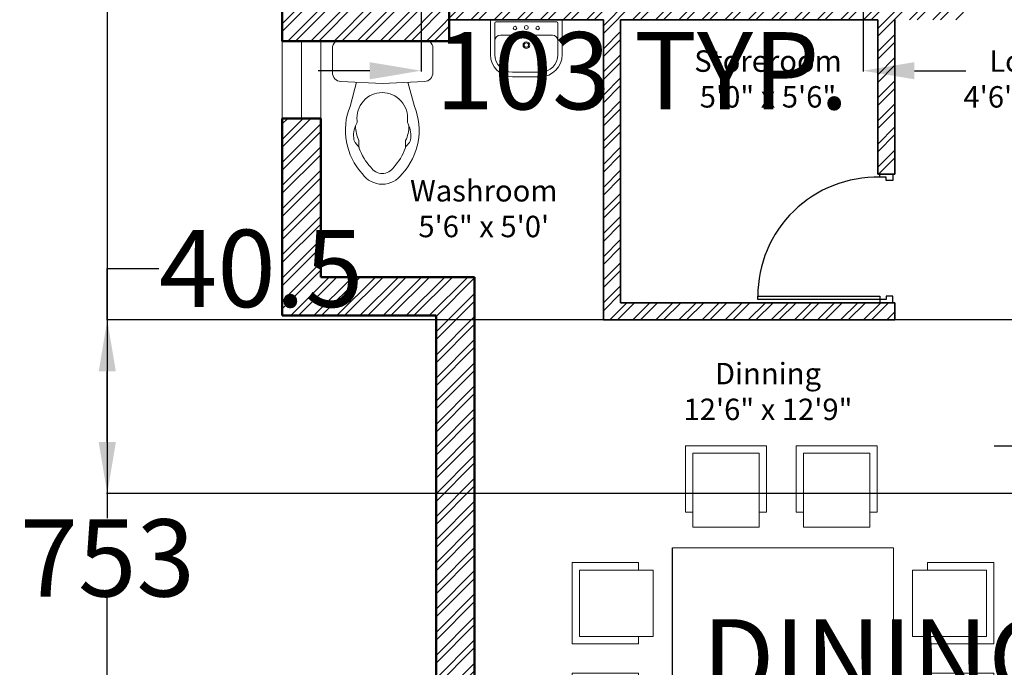
# Model space of a CAD drawing. Units: inches. Extents: x -90 to 536, y -553 to 299.
# Tile 15 of 27: x -23 to 207, y -153 to -2. Entities that reach past the tile are written whole.
import ezdxf

# ---------------------------------------------------------------- set-up
doc = ezdxf.new("R2010")
doc.units = ezdxf.units.IN
for name, color, linetype, lineweight in [('A-ANNO-DIMS', 2, 'Continuous', 18), ('A-AREA-IDEN', 7, 'Continuous', 18), ('A-DOOR', 4, 'Continuous', 25), ('A-FLOR-FIXT', 8, 'Continuous', 18), ('A-GLAZ', 4, 'Continuous', 18), ('A-WALL-PATT', 252, 'Continuous', 13), ('Furniture', 2, 'Continuous', 18), ('Inner Wall', 5, 'Continuous', 35), ('Outer Wall', 1, 'Continuous', 50)]:
    doc.layers.add(name, color=color, linetype=linetype, lineweight=lineweight)
doc.styles.get("Standard").update_dxf_attribs({"font": 'arial.ttf'})
doc.dimstyles.get("Standard").update_dxf_attribs({"dimtxt": 18, "dimasz": 12, "dimexe": 0.18, "dimexo": 0.0625, "dimgap": 0.09, "dimtad": 0, "dimtih": 1, "dimtoh": 1, "dimdec": 0, "dimzin": 0, "dimdsep": 46, "dimlunit": 3, "dimtxsty": 'Standard', "dimcen": 0.09, "dimadec": 0, "dimazin": 0, "dimtfac": 1, "dimtdec": 0, "dimtofl": 0, "dimtmove": 0, "dimatfit": 3, "dimfxl": 1, "dimtolj": 1, "dimtzin": 0, "dimarcsym": 0})

# ---------------------------------------------------------------- blocks, each defined once
blk = doc.blocks.new('A$C1308471B')
at = {"ltscale": 20}
for p, q in [((0.0354, 0.4793), (0.1495, 0.4793)), ((0, 0.4607), (0, 0.0186)), ((0.2013, 0.2397), (0.1923, 0.4384)), ((0.1957, 0.3639), (0.3109, 0.3953)), ((0.5021, 0.3528), (0.4724, 0.3528)), ((0.4982, 0.3575), (0.4822, 0.3709)), ((0.2013, 0.2397), (0.1923, 0.0409)), ((0.1959, 0.1193), (0.3109, 0.0879)), ((0.5021, 0.1304), (0.4724, 0.1304)), ((0.4982, 0.1257), (0.4822, 0.1123)), ((0.0354, 0), (0.1495, 0))]:
    blk.add_line(p, q, dxfattribs=at)
for centre, radius, start, end in [((0.0354, 0.4328), 0.0465, 90, 136.5269), ((0.1495, 0.4365), 0.0429, 2.5755, 90), ((0.006, 0.4607), 0.006, 136.5269, 180), ((0.4248, 0.1104), 0.3068, 47.4135, 111.7924), ((0.4494, 0.2636), 0.1148, 79.3968, 118.5742), ((0.4658, 0.3513), 0.0255, 50, 79.3968), ((0.3654, 0.2416), 0.1206, 83.3523, 180), ((0.3823, 0.3868), 0.0255, 263.3523, 298.5742), ((0.405, 0.2159), 0.153, 63.502, 90.4522), ((0.5146, 0.377), 0.0255, 230, 251.3881), ((0.5021, 0.3273), 0.0255, 70.3751, 90), ((0.4248, 0.1104), 0.2558, 46.612, 70.3751), ((0.5654, 0.2416), 0.116, 0, 54.7115), ((0.5654, 0.2416), 0.065, 0, 57.2974), ((0.3654, 0.2416), 0.1206, 180, 276.6477), ((0.5654, 0.2416), 0.065, 302.7026, 0), ((0.5654, 0.2416), 0.116, 305.2885, 0), ((0.4248, 0.3728), 0.3068, 248.2076, 312.5865), ((0.4248, 0.3728), 0.2558, 289.6249, 313.388), ((0.3823, 0.0964), 0.0255, 61.4258, 96.6477), ((0.4494, 0.2196), 0.1148, 241.4258, 280.6032), ((0.405, 0.2673), 0.153, 269.5478, 296.498), ((0.4658, 0.1319), 0.0255, 280.6032, 310), ((0.5146, 0.1062), 0.0255, 108.6119, 130), ((0.5021, 0.1559), 0.0255, 270, 289.6249), ((0.006, 0.0186), 0.006, 180, 223.4731), ((0.0354, 0.0465), 0.0465, 223.4731, 270), ((0.1495, 0.0429), 0.0429, 270, 357.4245)]:
    blk.add_arc(centre, radius, start, end, dxfattribs=at)
blk = doc.blocks.new('A$C57EA129C')
for p, q in [((0, 0.4428), (0, 0.1782)), ((0.016, 0.4589), (0.5631, 0.4589)), ((0.0356, 0.4321), (0.0356, 0.2896)), ((0.0445, 0.441), (0.5346, 0.441)), ((0.5435, 0.4321), (0.5435, 0.2896)), ((0.5791, 0.4428), (0.5791, 0.1782)), ((0.0802, 0.3341), (0.499, 0.3341)), ((0.0356, 0.2896), (0.0356, 0.1782)), ((0.5435, 0.2896), (0.5435, 0.1782)), ((0.1782, 0.0356), (0.4009, 0.0356)), ((0.1782, 0), (0.4009, 0))]:
    blk.add_line(p, q)
for centre, radius in [((0.1982, 0.392), 0.0143), ((0.2896, 0.3965), 0.0156), ((0.3809, 0.392), 0.0143), ((0.2896, 0.2545), 0.0267), ((0.2896, 0.2545), 0.0178)]:
    blk.add_circle(centre, radius)
for centre, radius, start, end in [((0.016, 0.4428), 0.016, 90, 180), ((0.0445, 0.4321), 0.00891, 90, 180), ((0.5346, 0.4321), 0.00891, 0, 90), ((0.5631, 0.4428), 0.016, 0, 90), ((0.0802, 0.2896), 0.0445, 90, 180), ((0.499, 0.2896), 0.0445, 0, 90), ((0.1782, 0.1782), 0.1782, 180, 270), ((0.1782, 0.1782), 0.1426, 180, 270), ((0.4009, 0.1782), 0.1782, 270, 0), ((0.4009, 0.1782), 0.1426, 270, 0)]:
    blk.add_arc(centre, radius, start, end)
blk = doc.blocks.new('A$C010165D4')
for p, q in [((0.7697, 2.4221), (0.7697, 2.8721)), ((0.7697, 2.8721), (1.3197, 2.8721)), ((1.3197, 2.8721), (1.3197, 2.4221)), ((1.5197, 2.4221), (1.5197, 2.8721)), ((1.5197, 2.8721), (2.0697, 2.8721)), ((2.0697, 2.8721), (2.0697, 2.4221)), ((0.8197, 2.8221), (0.8197, 2.3221)), ((1.2697, 2.8221), (0.8197, 2.8221)), ((1.2697, 2.3221), (1.2697, 2.8221)), ((1.5697, 2.8221), (1.5697, 2.3221)), ((2.0197, 2.8221), (1.5697, 2.8221)), ((2.0197, 2.3221), (2.0197, 2.8221)), ((0.8197, 2.4221), (0.7697, 2.4221)), ((1.3197, 2.4221), (1.2697, 2.4221)), ((1.5697, 2.4221), (1.5197, 2.4221)), ((2.0697, 2.4221), (2.0197, 2.4221)), ((1.2697, 2.3221), (0.8197, 2.3221)), ((2.0197, 2.3221), (1.5697, 2.3221)), ((0.6788, 2.1805), (0.6788, 0.6805)), ((0.6811, 0.6805), (0.6811, 2.1805)), ((0.6811, 2.1805), (2.1811, 2.1805)), ((2.1811, 2.1805), (2.1811, 0.6805)), ((0, 1.531), (0, 2.081)), ((0, 2.081), (0.45, 2.081)), ((0.45, 2.081), (0.45, 2.031)), ((2.8599, 2.081), (2.4099, 2.081)), ((2.4099, 2.081), (2.4099, 2.031)), ((2.8599, 1.531), (2.8599, 2.081)), ((0.05, 2.031), (0.05, 1.581)), ((0.55, 2.031), (0.05, 2.031)), ((0.55, 2.031), (0.55, 1.581)), ((2.3099, 2.031), (2.8099, 2.031)), ((2.3099, 2.031), (2.3099, 1.581)), ((2.8099, 2.031), (2.8099, 1.581)), ((0.05, 1.581), (0.55, 1.581)), ((0.45, 1.581), (0.45, 1.531)), ((2.8099, 1.581), (2.3099, 1.581)), ((2.4099, 1.581), (2.4099, 1.531)), ((0.45, 1.531), (0, 1.531)), ((2.4099, 1.531), (2.8599, 1.531)), ((0, 0.781), (0, 1.331)), ((0, 1.331), (0.45, 1.331)), ((0.05, 1.281), (0.05, 0.831)), ((0.55, 1.281), (0.05, 1.281)), ((0.45, 1.331), (0.45, 1.281)), ((0.55, 1.281), (0.55, 0.831)), ((2.3099, 1.281), (2.8099, 1.281)), ((2.3099, 1.281), (2.3099, 0.831)), ((2.4099, 1.331), (2.4099, 1.281)), ((2.8599, 1.331), (2.4099, 1.331)), ((2.8099, 1.281), (2.8099, 0.831)), ((2.8599, 0.781), (2.8599, 1.331)), ((0.05, 0.831), (0.55, 0.831)), ((0.45, 0.831), (0.45, 0.781)), ((2.8099, 0.831), (2.3099, 0.831)), ((2.4099, 0.831), (2.4099, 0.781)), ((0.45, 0.781), (0, 0.781)), ((2.4099, 0.781), (2.8599, 0.781)), ((2.1811, 0.6805), (0.6811, 0.6805)), ((0.8197, 0.05), (0.8197, 0.55)), ((1.2697, 0.55), (0.8197, 0.55)), ((1.2697, 0.55), (1.2697, 0.05)), ((1.5697, 0.05), (1.5697, 0.55)), ((2.0197, 0.55), (1.5697, 0.55)), ((2.0197, 0.55), (2.0197, 0.05)), ((0.7697, 0.45), (0.7697, 0)), ((0.8197, 0.45), (0.7697, 0.45)), ((1.3197, 0.45), (1.2697, 0.45)), ((1.3197, 0), (1.3197, 0.45)), ((1.5197, 0.45), (1.5197, 0)), ((1.5697, 0.45), (1.5197, 0.45)), ((2.0697, 0.45), (2.0197, 0.45)), ((2.0697, 0), (2.0697, 0.45)), ((1.2697, 0.05), (0.8197, 0.05)), ((2.0197, 0.05), (1.5697, 0.05)), ((0.7697, 0), (1.3197, 0)), ((1.5197, 0), (2.0697, 0))]:
    blk.add_line(p, q)
blk = doc.blocks.new('*D34')
at = {"layer": 'A-ANNO-DIMS', "color": 0, "lineweight": -2, "transparency": 16777216}
for p, q in [((70.57, 2.38), (70.57, -13.63)), ((173.7, 2.38), (173.7, -13.63)), ((58.57, -13.45), (46.57, -13.45)), ((185.7, -13.45), (197.7, -13.45))]:
    blk.add_line(p, q, dxfattribs=at)
at = {"layer": 'A-ANNO-DIMS', "color": 0, "transparency": 16777216}
for points in [[(58.57, -11.45), (58.57, -15.45), (70.57, -13.45)], [(185.7, -11.45), (185.7, -15.45), (173.7, -13.45)]]:
    blk.add_solid(points, dxfattribs=at)
at = {"layer": 'Defpoints', "color": 0, "transparency": 16777216}
for p in [(70.57, 2.45), (173.7, 2.45), (70.57, -13.45)]:
    blk.add_point(p, dxfattribs=at)
at = {"layer": 'A-ANNO-DIMS', "color": 0, "transparency": 16777216, "insert": (122.13, -13.45), "char_height": 18, "attachment_point": 5}
blk.add_mtext('\\A1;103 TYP.', dxfattribs=at)
blk = doc.blocks.new('*D41')
at = {"layer": 'A-ANNO-DIMS', "color": 0, "lineweight": -2, "transparency": 16777216}
for p, q in [((204.27, -100.92), (219.21, -100.92)), ((219.03, -112.92), (219.03, -140.95)), ((219.03, -187.77), (219.03, -159.74)), ((204.27, -199.77), (219.21, -199.77))]:
    blk.add_line(p, q, dxfattribs=at)
at = {"layer": 'A-ANNO-DIMS', "color": 0, "transparency": 16777216}
for points in [[(217.03, -112.92), (221.03, -112.92), (219.03, -100.92)], [(217.03, -187.77), (221.03, -187.77), (219.03, -199.77)]]:
    blk.add_solid(points, dxfattribs=at)
at = {"layer": 'Defpoints', "color": 0, "transparency": 16777216}
for p in [(204.21, -100.92), (219.03, -100.92), (204.21, -199.77)]:
    blk.add_point(p, dxfattribs=at)
at = {"layer": 'A-ANNO-DIMS', "color": 0, "transparency": 16777216, "insert": (219.03, -150.34), "char_height": 18, "attachment_point": 5}
blk.add_mtext('\\A1;DINING SET 99', dxfattribs=at)
blk = doc.blocks.new('*D53')
at = {"layer": 'A-ANNO-DIMS', "color": 0, "lineweight": -2, "transparency": 16777216}
for p, q in [((35.09, 103.75), (35.09, 287.38)), ((407.13, -63.49), (407.13, 287.38)), ((47.09, 287.2), (183.7, 287.2)), ((395.13, 287.2), (258.52, 287.2))]:
    blk.add_line(p, q, dxfattribs=at)
at = {"layer": 'A-ANNO-DIMS', "color": 0, "transparency": 16777216}
for points in [[(47.09, 289.2), (47.09, 285.2), (35.09, 287.2)], [(395.13, 289.2), (395.13, 285.2), (407.13, 287.2)]]:
    blk.add_solid(points, dxfattribs=at)
at = {"layer": 'Defpoints', "color": 0, "transparency": 16777216}
for p in [(407.13, 287.2), (35.09, 103.69), (407.13, -63.55)]:
    blk.add_point(p, dxfattribs=at)
at = {"layer": 'A-ANNO-DIMS', "color": 0, "transparency": 16777216, "insert": (221.11, 287.2), "char_height": 18, "attachment_point": 5}
blk.add_mtext('\\A1;372.04', dxfattribs=at)
blk = doc.blocks.new('*D54')
at = {"layer": 'A-ANNO-DIMS', "color": 0, "lineweight": -2, "transparency": 16777216}
for p, q in [((113.07, 249.45), (-2.85, 249.45)), ((-2.67, 237.45), (-2.67, -117.77)), ((-2.67, -491.55), (-2.67, -136.34)), ((38.07, -503.55), (-2.85, -503.55))]:
    blk.add_line(p, q, dxfattribs=at)
at = {"layer": 'A-ANNO-DIMS', "color": 0, "transparency": 16777216}
for points in [[(-4.67, 237.45), (-0.67, 237.45), (-2.67, 249.45)], [(-4.67, -491.55), (-0.67, -491.55), (-2.67, -503.55)]]:
    blk.add_solid(points, dxfattribs=at)
at = {"layer": 'Defpoints', "color": 0, "transparency": 16777216}
for p in [(-2.67, 249.45), (113.13, 249.45), (38.13, -503.55)]:
    blk.add_point(p, dxfattribs=at)
at = {"layer": 'A-ANNO-DIMS', "color": 0, "transparency": 16777216, "insert": (-2.67, -127.05), "char_height": 18, "attachment_point": 5}
blk.add_mtext('\\A1;753', dxfattribs=at)
blk = doc.blocks.new('*D60')
at = {"layer": 'A-ANNO-DIMS', "color": 0, "lineweight": -2, "transparency": 16777216}
for p, q in [((-2.67, -71.55), (-2.67, -59.55)), ((-2.67, -59.55), (9.33, -59.55)), ((290.07, -71.55), (-2.85, -71.55)), ((-2.67, -100.05), (-2.67, -83.55)), ((290.07, -112.05), (-2.85, -112.05))]:
    blk.add_line(p, q, dxfattribs=at)
at = {"layer": 'A-ANNO-DIMS', "color": 0, "transparency": 16777216}
for points in [[(-4.67, -83.55), (-0.67, -83.55), (-2.67, -71.55)], [(-4.67, -100.05), (-0.67, -100.05), (-2.67, -112.05)]]:
    blk.add_solid(points, dxfattribs=at)
at = {"layer": 'Defpoints', "color": 0, "transparency": 16777216}
for p in [(-2.67, -71.55), (290.13, -71.55), (290.13, -112.05)]:
    blk.add_point(p, dxfattribs=at)
at = {"layer": 'A-ANNO-DIMS', "color": 0, "transparency": 16777216, "insert": (33.23, -59.55), "char_height": 18, "attachment_point": 5}
blk.add_mtext('\\A1;40.5', dxfattribs=at)

msp = doc.modelspace()

# ---------------------------------------------------------------- hatches: boundary and pattern name
at = {"layer": 'A-WALL-PATT'}
h = msp.add_hatch(dxfattribs=at)
h.set_pattern_fill('ANSI32', color=256, scale=0.4)
h.set_pattern_definition([(45, (-88.8105, -603.6155), (-2.694077, 2.694077), []), (45, (-87.0145, -603.6155), (-2.694077, 2.694077), [])])
h.paths.add_polyline_path([(285.1317, 246.4462), (131.1317, 246.4462), (131.1317, 237.4462), (285.1317, 237.4462)])
h.paths.add_polyline_path([(122.1317, 237.4462), (113.1317, 237.4462), (113.1317, 152.4462), (122.1317, 152.4462), (122.1317, 166.4704)])
h.paths.add_polyline_path([(303.1317, 237.4462), (294.1317, 237.4462), (294.1317, 152.4462), (303.1317, 152.4462)])
h.paths.add_polyline_path([(47.1317, 91.9277), (38.1317, 91.9277), (38.1317, -6.5538), (77.1317, -6.5538), (77.1317, 2.4462), (70.5655, 2.4462), (47.1317, 2.4462)])
h.paths.add_polyline_path([(83.052, -61.5538), (47.1317, -61.5538), (47.1317, -24.5538), (38.1317, -24.5538), (38.1317, -70.5538), (74.052, -70.5538), (74.052, -223.5538), (38.1317, -223.5538), (38.1317, -503.5538), (92.1317, -503.5538), (92.1317, -437.5538), (191.1317, -437.5538), (191.1317, -428.5538), (83.1317, -428.5538), (83.1317, -494.5538), (47.1317, -494.5538), (47.1317, -232.5538), (83.052, -232.5538), (83.052, -70.5538)])
h.paths.add_polyline_path([(407.1317, -63.5538), (381.1317, -63.5538), (381.1317, 91.9277), (372.1317, 91.9277), (372.1317, 32.8805), (372.1317, -63.5538), (306.5745, -63.5538), (237.1317, -63.5538), (237.1317, -38.5538), (233.1317, -38.5538), (233.1317, -71.5538), (398.1317, -71.5538), (398.1317, -152.5538), (233.1317, -152.5538), (233.1317, -161.5538), (398.1317, -161.5538), (398.1317, -368.5538), (233.1317, -368.5538), (233.1317, -377.5538), (407.1317, -377.5538), (407.1317, -161.5538)])
h.paths.add_polyline_path([(261.1317, -422.5538), (252.1317, -422.5538), (252.1317, -428.5538), (233.1317, -428.5538), (233.1317, -437.5538), (261.1317, -437.5538)])
h.paths.add_polyline_path([(191.1317, -368.5538), (180.1317, -368.5538), (180.1317, -335.5538), (131.5919, -335.5538), (131.5919, -344.5538), (171.1317, -344.5538), (171.1317, -392.5538), (180.1317, -392.5538), (180.1317, -377.5538), (191.1317, -377.5538)], flags=17)
h.paths.add_polyline_path([(180.1317, -223.5538), (152.1317, -223.5538), (152.1317, -227.5538), (176.1317, -227.5538), (176.1317, -335.5538), (180.1317, -335.5538)], flags=17)
h.paths.add_polyline_path([(131.5919, -335.5538), (83.1317, -335.5538), (83.1317, -339.5538), (83.1317, -392.5538), (87.1317, -392.5538), (87.1317, -339.5538), (131.5919, -339.5538)], flags=17)
h.paths.add_polyline_path([(197.1317, 2.4462), (77.1317, 2.4462), (77.1317, -1.5538), (113.1317, -1.5538), (113.1317, -71.5538), (181.1317, -71.5538), (181.1317, -67.5538), (117.1317, -67.5538), (117.1317, -1.5538), (177.1317, -1.5538), (177.1317, -37.5538), (181.1317, -37.5538), (181.1317, -1.5538), (197.1317, -1.5538)])
h.paths.add_polyline_path([(173.1317, 138.4462), (122.1317, 138.4462), (122.1317, 134.4462), (173.1317, 134.4462)])
h.paths.add_polyline_path([(213.1317, 237.4462), (209.1317, 237.4462), (209.1317, 134.4462), (233.1317, 134.4462), (233.1317, 68.8889), (233.1317, -2.5538), (237.1317, -2.5538), (237.1317, 134.4462), (258.1317, 134.4462), (258.1317, 138.4462), (213.1317, 138.4462)])

# ---------------------------------------------------------------- linework, layer by layer
at = {"layer": 'A-DOOR'}
for points in [[(180.6317, -37.5538), (180.6317, -39.0538), (179.1317, -39.0538), (179.1317, -38.3038), (177.6317, -38.3038), (177.6317, -37.5538)], [(149.1317, -66.8038), (149.1317, -66.0538), (177.6317, -66.0538), (177.6317, -66.8038)], [(180.6317, -67.5538), (180.6317, -66.0538), (179.1317, -66.0538), (179.1317, -66.8038), (177.6317, -66.8038), (177.6317, -67.5538)]]:
    msp.add_lwpolyline(points, close=True, dxfattribs=at)
msp.add_arc((176.8916, -66.0538), 27.7599, 88.472203, 180, dxfattribs=at)
at = {"layer": 'A-GLAZ'}
for p, q in [((38.1317, -24.5538), (38.1317, -6.5538)), ((42.6317, -24.5538), (42.6317, -6.5538)), ((47.1317, -24.5538), (47.1317, -6.5538))]:
    msp.add_line(p, q, dxfattribs=at)
at = {"layer": 'Inner Wall'}
for p, q in [((113.1317, -1.5538), (77.1317, -1.5538)), ((113.1317, -1.5538), (113.1317, -71.5538)), ((117.1317, -1.5538), (117.1317, -67.5538)), ((177.1317, -1.5538), (117.1317, -1.5538)), ((177.1317, -1.5538), (177.1317, -37.5538)), ((181.1317, -1.5538), (181.1317, -37.5538)), ((181.1317, -37.5538), (177.1317, -37.5538)), ((181.1317, -67.5538), (117.1317, -67.5538)), ((181.1317, -67.5538), (181.1317, -71.5538)), ((181.1317, -71.5538), (113.1317, -71.5538))]:
    msp.add_line(p, q, dxfattribs=at)
at = {"layer": 'Outer Wall'}
for p, q in [((38.1317, 91.9277), (38.1317, -6.5538)), ((77.1317, 2.4462), (77.1317, -6.5538)), ((77.1317, -6.5538), (38.1317, -6.5538)), ((47.1317, -24.5538), (38.1317, -24.5538)), ((38.1317, -24.5538), (38.1317, -70.5538)), ((47.1317, -24.5538), (47.1317, -61.5538)), ((83.052, -61.5538), (47.1317, -61.5538)), ((83.052, -61.5538), (83.052, -70.5538)), ((74.052, -70.5538), (38.1317, -70.5538)), ((74.052, -70.5538), (74.052, -223.5538)), ((83.052, -70.5538), (83.052, -232.5538))]:
    msp.add_line(p, q, dxfattribs=at)

# ---------------------------------------------------------------- block references
at = {"layer": 'A-FLOR-FIXT', "xscale": 28.98333223671166, "yscale": 28.98333223671166, "zscale": 28.98333223671166}
msp.add_blockref('A$C57EA129C', (86.7389, -14.8532), dxfattribs=at)
at = {"layer": 'A-FLOR-FIXT', "xscale": -48.95497407897215, "yscale": 48.95497407897215, "zscale": 48.95497407897215, "rotation": 90}
msp.add_blockref('A$C1308471B', (73.3267, -6.5538), dxfattribs=at)
at = {"layer": 'Furniture', "xscale": 34.41518617011034, "yscale": 34.41518617011034, "zscale": 34.41518617011034}
msp.add_blockref('A$C010165D4', (105.7848, -199.766), dxfattribs=at)

# ---------------------------------------------------------------- texts
at = {"layer": 'A-AREA-IDEN', "char_height": 5, "attachment_point": 3}
for s, insert in [('\\pxqc;{\\fTimes New Roman|b0|i0|c0|p18;Storeroom\\P5\'0" x 5\'6"}', (176.1952, -8.7077)), ('\\pxqc;{\\fTimes New Roman|b0|i0|c0|p18;Lobby\\P4\'6" x 5\'9"}', (237.7373, -8.7077)), ('\\pxqc;{\\fTimes New Roman|b0|i0|c0|p18;Washroom\\P5\'6" x 5\'0\'}', (109.8578, -38.9395)), ('\\pxqc;{\\fTimes New Roman|b0|i0|c0|p18;Dinning\\P12\'6" x 12\'9"}', (176.1952, -81.577))]:
    msp.add_mtext_dynamic_manual_height_columns(s, width=49.342153, gutter_width=12.5, heights=[0], dxfattribs=dict(at, insert=insert))

# ---------------------------------------------------------------- dimensions: what is measured, and where the dimension line sits
at = {"layer": 'A-ANNO-DIMS'}
dim = msp.add_linear_dim(base=(407.1317, 287.2012), p1=(35.0873, 103.6916), p2=(407.1317, -63.5538), dimstyle='Standard', override={"dimdec": 2, "dimlfac": 1, "dimrnd": 0, "dimzin": 0, "dimdsep": 46, "dimlunit": 2}, dxfattribs=at)
dim.commit()
dim.dimension.update_dxf_attribs({"geometry": '*D53', "text_midpoint": (221.1095, 287.2012)})
for base, p1, p2, override, picture, middle in [((-2.6677, 249.4462), (38.1317, -503.5538), (113.1317, 249.4462), {"dimdec": 0, "dimlfac": 1, "dimrnd": 0, "dimzin": 0, "dimdsep": 46, "dimlunit": 2}, '*D54', (-2.6677, -127.0538)), ((-2.6677, -71.5538), (290.1317, -112.0538), (290.1317, -71.5538), {"dimdec": 1, "dimlfac": 1, "dimrnd": 0, "dimzin": 0, "dimdsep": 46, "dimlunit": 2}, '*D60', (33.2299, -59.5538))]:
    dim = msp.add_linear_dim(base=base, p1=p1, p2=p2, angle=90, dimstyle='Standard', override=override, dxfattribs=at)
    dim.commit()
    dim.dimension.update_dxf_attribs({"geometry": picture, "text_midpoint": middle})
for base, p1, p2, angle, text, picture, middle in [((70.5655, -13.447), (173.698, 2.4462), (70.5655, 2.4462), 180, '<> TYP.', '*D34', (122.1317, -13.447)), ((219.0345, -100.9205), (204.2077, -199.766), (204.2077, -100.9205), 90, 'DINING SET <>', '*D41', (219.0345, -150.3432))]:
    dim = msp.add_linear_dim(base=base, p1=p1, p2=p2, angle=angle, text=text, dimstyle='Standard', override={"dimdec": 0, "dimlfac": 1, "dimrnd": 0, "dimzin": 0, "dimdsep": 46, "dimlunit": 2}, dxfattribs=at)
    dim.commit()
    dim.dimension.update_dxf_attribs({"geometry": picture, "text_midpoint": middle})

doc.saveas('drawing.dxf')
